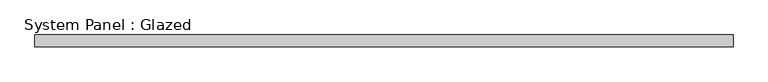
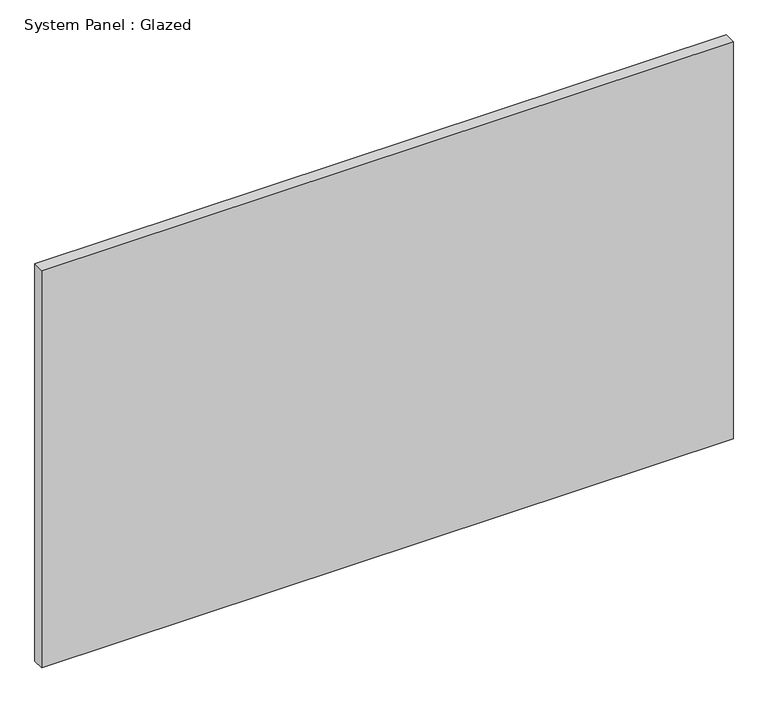
"""IFC4 building model written with IfcOpenShell, lengths in millimetres: plate geometry, System Panel : Glazed."""

from ifc_helpers import new_model, si_unit, origin, origin_with_axes, place, context, project, spatial, polyline, outline, extrude, source, transform, mapped, element, save


def system_panel_glazed_b07a1a35(model_context):
    return source(origin(), model_context, "Body", "SweptSolid", [
        extrude(outline(polyline([(752.6151949, 19.05), (-752.6151949, 19.05), (-752.6151949, 44.45), (752.6151949, 44.45), (752.6151949, 19.05)])), origin_with_axes(), (0.0, 0.0, 1.0), 914.4),
    ])


if __name__ == "__main__":
    model = new_model("IFC4")
    model_context = context("Model", 3, world=origin())
    ifc_project = project(units=[si_unit("LENGTHUNIT", "METRE", prefix="MILLI")], contexts=[model_context])
    site = spatial("IfcSite", under=ifc_project)
    building = spatial("IfcBuilding", under=site)
    placement = place(None, origin())
    system_panel_glazed_shape = system_panel_glazed_b07a1a35(model_context)
    element("IfcPlate", 1, ObjectType="System Panel : Glazed", at=placement, inside=building, context=model_context, shape_type="MappedRepresentation", body=[
        mapped(system_panel_glazed_shape, transform((0.0, 0.0, 0.0), x_axis=(1.0, 0.0, 0.0), y_axis=(0.0, 1.0, 0.0), z_axis=(0.0, 0.0, 1.0))),
    ])
    save(model, "model.ifc")

# Revit data of these elements
# Type "System Panel : Glazed"
#   Construction Type Id = "GSP4R"
#   Analytic Construction = "1/8 in Pilkington single glazing"
#   Visual Light Transmittance = 0.9
#   Solar Heat Gain Coefficient = 0.86
#   Heat Transfer Coefficient (U) = 6.7069 W/(m²·K)
# Element 1 (IfcPlate, "System Panel : Glazed")
#   Materials on its faces: "Glass"
# Materials
#   "Glass": class "Glass", colour RGB 0 128 192, transparency 0.75, Description = "Soda Lime Glass", Cost = 0
